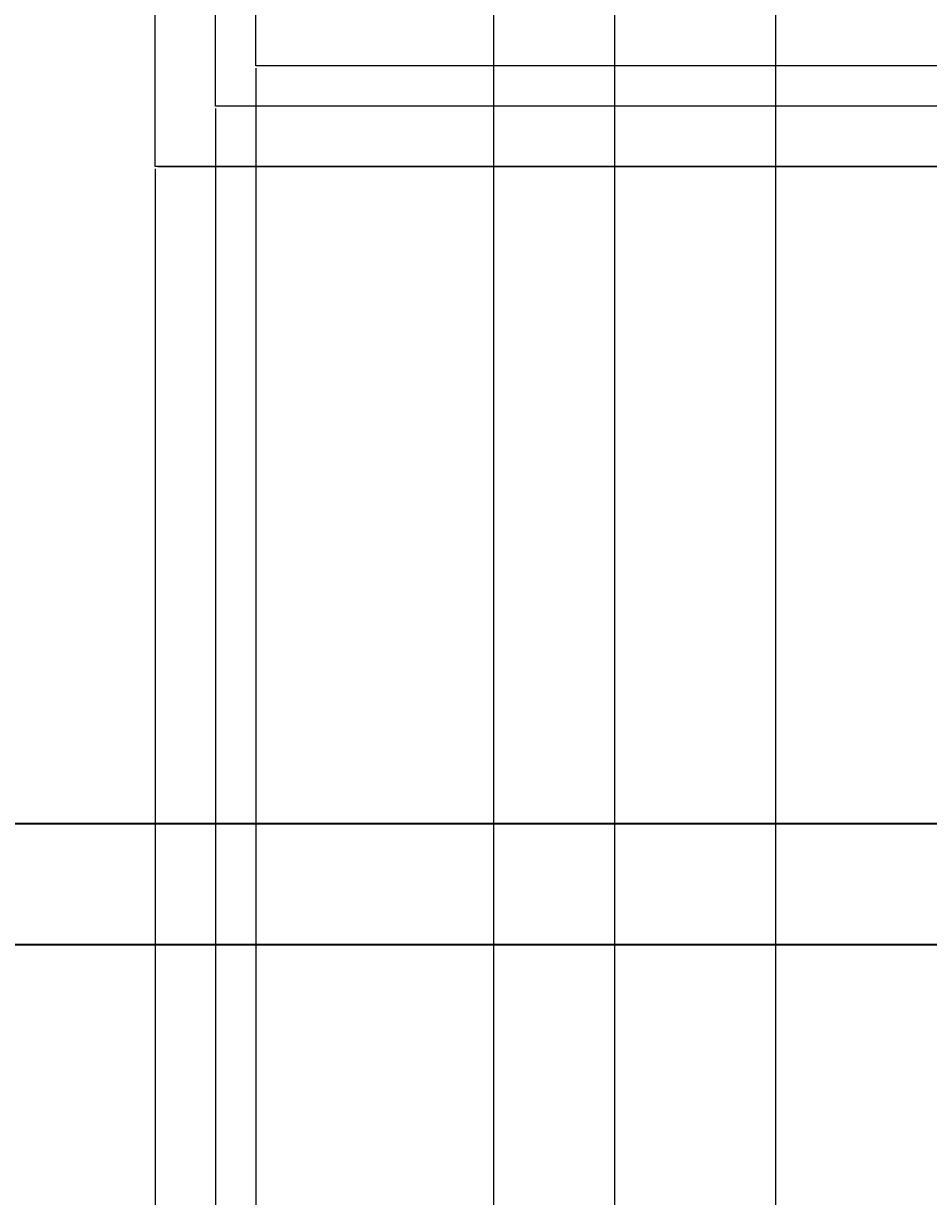
# Model space of a CAD drawing. Units: inches. Extents: x -6 to 289, y -8 to 323.
# Tile 51 of 107: x 124 to 146, y 153 to 182. Entities that reach past the tile are written whole.
import ezdxf

# ---------------------------------------------------------------- set-up
doc = ezdxf.new("R2010")
doc.units = ezdxf.units.IN
doc.header["$MEASUREMENT"] = 0
for name, color, linetype, lineweight in [('A-ANNO-DIMS', 2, 'Continuous', 18), ('A-ELEV', 7, 'Continuous', 35), ('A-ELEV-PATT', 8, 'Continuous', 13), ('A-GLAZ', 4, 'Continuous', 25)]:
    doc.layers.add(name, color=color, linetype=linetype, lineweight=lineweight)
doc.styles.get("Standard").update_dxf_attribs({"font": 'arial.ttf'})
doc.dimstyles.get("Standard").update_dxf_attribs({"dimtxt": 0.18, "dimasz": 0.18, "dimexe": 0.18, "dimexo": 0.0625, "dimgap": 0.09, "dimtad": 0, "dimtih": 1, "dimtoh": 1, "dimdec": 4, "dimzin": 0, "dimdsep": 46, "dimtxsty": 'Standard', "dimcen": 0.09, "dimadec": 0, "dimazin": 0, "dimtfac": 1, "dimtdec": 4, "dimtofl": 0, "dimtmove": 0, "dimatfit": 3, "dimfxl": 1, "dimtolj": 1, "dimtzin": 0, "dimarcsym": 0})

# ---------------------------------------------------------------- blocks, each defined once
blk = doc.blocks.new('*U4')
for p, q in [((1.5, 1.5), (1.5, 46.5)), ((21, 1.5), (1.5, 1.5))]:
    blk.add_line(p, q)
blk.add_lwpolyline([(0, 0), (0, 48), (42, 48), (42, 0)], close=True)
blk.add_lwpolyline([(20, 45.5), (20, 2.5), (2.5, 2.5), (2.5, 45.5), (20, 45.5)])
blk = doc.blocks.new('*D24')
at = {"layer": 'A-ANNO-DIMS', "color": 0, "lineweight": -2, "transparency": 16777216}
for p, q in [((126.946, 178.654), (288.653, 178.654)), ((288.473, 178.474), (288.473, 159.153)), ((288.473, 139.469), (288.473, 158.789)), ((259.226, 139.289), (288.653, 139.289))]:
    blk.add_line(p, q, dxfattribs=at)
at = {"layer": 'A-ANNO-DIMS', "color": 0, "transparency": 16777216}
for points in [[(288.443, 178.474), (288.503, 178.474), (288.473, 178.654)], [(288.443, 139.469), (288.503, 139.469), (288.473, 139.289)]]:
    blk.add_solid(points, dxfattribs=at)
at = {"layer": 'Defpoints', "color": 0, "transparency": 16777216}
for p in [(126.883, 178.654), (288.473, 178.654), (259.164, 139.289)]:
    blk.add_point(p, dxfattribs=at)
at = {"layer": 'A-ANNO-DIMS', "color": 0, "transparency": 16777216, "insert": (288.473, 158.971), "char_height": 0.18, "attachment_point": 5}
blk.add_mtext('\\A1;39.365', dxfattribs=at)
blk = doc.blocks.new('*D25')
at = {"layer": 'A-ANNO-DIMS', "color": 0, "lineweight": -2, "transparency": 16777216}
for p, q in [((126.946, 226.654), (288.653, 226.654)), ((288.473, 226.474), (288.473, 202.836)), ((288.473, 178.834), (288.473, 202.472)), ((126.946, 178.654), (288.653, 178.654))]:
    blk.add_line(p, q, dxfattribs=at)
at = {"layer": 'A-ANNO-DIMS', "color": 0, "transparency": 16777216}
for points in [[(288.443, 226.474), (288.503, 226.474), (288.473, 226.654)], [(288.443, 178.834), (288.503, 178.834), (288.473, 178.654)]]:
    blk.add_solid(points, dxfattribs=at)
at = {"layer": 'Defpoints', "color": 0, "transparency": 16777216}
for p in [(126.883, 226.654), (288.473, 226.654), (126.883, 178.654)]:
    blk.add_point(p, dxfattribs=at)
at = {"layer": 'A-ANNO-DIMS', "color": 0, "transparency": 16777216, "insert": (288.473, 202.654), "char_height": 0.18, "attachment_point": 5}
blk.add_mtext('\\A1;48', dxfattribs=at)
blk = doc.blocks.new('*D28')
at = {"layer": 'A-ANNO-DIMS', "color": 0, "lineweight": -2, "transparency": 16777216}
for p, q in [((128.383, 180.092), (128.383, -8.391)), ((126.883, 178.592), (126.883, -8.391)), ((127.063, -8.211), (127.387, -8.211)), ((128.203, -8.211), (127.88, -8.211))]:
    blk.add_line(p, q, dxfattribs=at)
at = {"layer": 'A-ANNO-DIMS', "color": 0, "transparency": 16777216}
for points in [[(127.063, -8.181), (127.063, -8.241), (126.883, -8.211)], [(128.203, -8.181), (128.203, -8.241), (128.383, -8.211)]]:
    blk.add_solid(points, dxfattribs=at)
at = {"layer": 'Defpoints', "color": 0, "transparency": 16777216}
for p in [(128.383, 180.154), (126.883, 178.654), (128.383, -8.211)]:
    blk.add_point(p, dxfattribs=at)
at = {"layer": 'A-ANNO-DIMS', "color": 0, "transparency": 16777216, "insert": (127.633, -8.211), "char_height": 0.18, "attachment_point": 5}
blk.add_mtext('\\A1;1.5', dxfattribs=at)
blk = doc.blocks.new('*D29')
at = {"layer": 'A-ANNO-DIMS', "color": 0, "lineweight": -2, "transparency": 16777216}
for p, q in [((129.383, 181.092), (129.383, -8.391)), ((128.383, 180.092), (128.383, -8.391)), ((128.563, -8.211), (128.76, -8.211)), ((129.203, -8.211), (129.007, -8.211))]:
    blk.add_line(p, q, dxfattribs=at)
at = {"layer": 'A-ANNO-DIMS', "color": 0, "transparency": 16777216}
for points in [[(128.563, -8.181), (128.563, -8.241), (128.383, -8.211)], [(129.203, -8.181), (129.203, -8.241), (129.383, -8.211)]]:
    blk.add_solid(points, dxfattribs=at)
at = {"layer": 'Defpoints', "color": 0, "transparency": 16777216}
for p in [(129.383, 181.154), (128.383, 180.154), (129.383, -8.211)]:
    blk.add_point(p, dxfattribs=at)
at = {"layer": 'A-ANNO-DIMS', "color": 0, "transparency": 16777216, "insert": (128.883, -8.211), "char_height": 0.18, "attachment_point": 5}
blk.add_mtext('\\A1;1', dxfattribs=at)
blk = doc.blocks.new('*D30')
at = {"layer": 'A-ANNO-DIMS', "color": 0, "lineweight": -2, "transparency": 16777216}
for p, q in [((129.383, 181.092), (129.383, -8.391)), ((146.883, 181.092), (146.883, -8.391)), ((129.563, -8.211), (137.817, -8.211)), ((146.703, -8.211), (138.449, -8.211))]:
    blk.add_line(p, q, dxfattribs=at)
at = {"layer": 'A-ANNO-DIMS', "color": 0, "transparency": 16777216}
for points in [[(129.563, -8.181), (129.563, -8.241), (129.383, -8.211)], [(146.703, -8.181), (146.703, -8.241), (146.883, -8.211)]]:
    blk.add_solid(points, dxfattribs=at)
at = {"layer": 'Defpoints', "color": 0, "transparency": 16777216}
for p in [(129.383, 181.154), (146.883, 181.154), (146.883, -8.211)]:
    blk.add_point(p, dxfattribs=at)
at = {"layer": 'A-ANNO-DIMS', "color": 0, "transparency": 16777216, "insert": (138.133, -8.211), "char_height": 0.18, "attachment_point": 5}
blk.add_mtext('\\A1;17.5', dxfattribs=at)
blk = doc.blocks.new('*D73')
at = {"layer": 'A-ANNO-DIMS', "color": 0, "lineweight": -2, "transparency": 16777216}
for p, q in [((121.008, 51.148), (121.008, 322.969)), ((135.296, 51.148), (135.296, 322.969)), ((121.188, 322.789), (127.697, 322.789)), ((135.116, 322.789), (128.607, 322.789))]:
    blk.add_line(p, q, dxfattribs=at)
at = {"layer": 'A-ANNO-DIMS', "color": 0, "transparency": 16777216}
for points in [[(121.188, 322.819), (121.188, 322.759), (121.008, 322.789)], [(135.116, 322.819), (135.116, 322.759), (135.296, 322.789)]]:
    blk.add_solid(points, dxfattribs=at)
at = {"layer": 'Defpoints', "color": 0, "transparency": 16777216}
for p in [(135.296, 322.789), (121.008, 51.085), (135.296, 51.085)]:
    blk.add_point(p, dxfattribs=at)
at = {"layer": 'A-ANNO-DIMS', "color": 0, "transparency": 16777216, "insert": (128.152, 322.789), "char_height": 0.18, "attachment_point": 5}
blk.add_mtext('\\A1;14.288', dxfattribs=at)
blk = doc.blocks.new('*D74')
at = {"layer": 'A-ANNO-DIMS', "color": 0, "lineweight": -2, "transparency": 16777216}
for p, q in [((135.296, 51.148), (135.296, 322.969)), ((138.296, 51.148), (138.296, 322.969)), ((135.476, 322.789), (136.647, 322.789)), ((138.116, 322.789), (136.945, 322.789))]:
    blk.add_line(p, q, dxfattribs=at)
at = {"layer": 'A-ANNO-DIMS', "color": 0, "transparency": 16777216}
for points in [[(135.476, 322.819), (135.476, 322.759), (135.296, 322.789)], [(138.116, 322.819), (138.116, 322.759), (138.296, 322.789)]]:
    blk.add_solid(points, dxfattribs=at)
at = {"layer": 'Defpoints', "color": 0, "transparency": 16777216}
for p in [(138.296, 322.789), (135.296, 51.085), (138.296, 51.085)]:
    blk.add_point(p, dxfattribs=at)
at = {"layer": 'A-ANNO-DIMS', "color": 0, "transparency": 16777216, "insert": (136.796, 322.789), "char_height": 0.18, "attachment_point": 5}
blk.add_mtext('\\A1;3', dxfattribs=at)
blk = doc.blocks.new('*D75')
at = {"layer": 'A-ANNO-DIMS', "color": 0, "lineweight": -2, "transparency": 16777216}
for p, q in [((138.296, 51.148), (138.296, 322.969)), ((142.296, 51.148), (142.296, 322.969)), ((138.476, 322.789), (140.144, 322.789)), ((142.116, 322.789), (140.448, 322.789))]:
    blk.add_line(p, q, dxfattribs=at)
at = {"layer": 'A-ANNO-DIMS', "color": 0, "transparency": 16777216}
for points in [[(138.476, 322.819), (138.476, 322.759), (138.296, 322.789)], [(142.116, 322.819), (142.116, 322.759), (142.296, 322.789)]]:
    blk.add_solid(points, dxfattribs=at)
at = {"layer": 'Defpoints', "color": 0, "transparency": 16777216}
for p in [(142.296, 322.789), (138.296, 51.085), (142.296, 51.085)]:
    blk.add_point(p, dxfattribs=at)
at = {"layer": 'A-ANNO-DIMS', "color": 0, "transparency": 16777216, "insert": (140.296, 322.789), "char_height": 0.18, "attachment_point": 5}
blk.add_mtext('\\A1;4', dxfattribs=at)
blk = doc.blocks.new('*D76')
at = {"layer": 'A-ANNO-DIMS', "color": 0, "lineweight": -2, "transparency": 16777216}
for p, q in [((142.296, 51.148), (142.296, 322.969)), ((164.296, 51.148), (164.296, 322.969)), ((142.476, 322.789), (153.076, 322.789)), ((164.116, 322.789), (153.516, 322.789))]:
    blk.add_line(p, q, dxfattribs=at)
at = {"layer": 'A-ANNO-DIMS', "color": 0, "transparency": 16777216}
for points in [[(142.476, 322.819), (142.476, 322.759), (142.296, 322.789)], [(164.116, 322.819), (164.116, 322.759), (164.296, 322.789)]]:
    blk.add_solid(points, dxfattribs=at)
at = {"layer": 'Defpoints', "color": 0, "transparency": 16777216}
for p in [(164.296, 322.789), (142.296, 51.085), (164.296, 51.085)]:
    blk.add_point(p, dxfattribs=at)
at = {"layer": 'A-ANNO-DIMS', "color": 0, "transparency": 16777216, "insert": (153.296, 322.789), "char_height": 0.18, "attachment_point": 5}
blk.add_mtext('\\A1;22', dxfattribs=at)
blk = doc.blocks.new('*D94')
at = {"layer": 'A-ANNO-DIMS', "color": 0, "lineweight": -2, "transparency": 16777216}
for p, q in [((118.164, 159.411), (118.164, 322.969)), ((161.552, 159.411), (161.552, 322.969)), ((118.344, 322.789), (139.46, 322.789)), ((161.372, 322.789), (140.256, 322.789))]:
    blk.add_line(p, q, dxfattribs=at)
at = {"layer": 'A-ANNO-DIMS', "color": 0, "transparency": 16777216}
for points in [[(118.344, 322.819), (118.344, 322.759), (118.164, 322.789)], [(161.372, 322.819), (161.372, 322.759), (161.552, 322.789)]]:
    blk.add_solid(points, dxfattribs=at)
at = {"layer": 'Defpoints', "color": 0, "transparency": 16777216}
for p in [(161.552, 322.789), (118.164, 159.348), (161.552, 159.348)]:
    blk.add_point(p, dxfattribs=at)
at = {"layer": 'A-ANNO-DIMS', "color": 0, "transparency": 16777216, "insert": (139.858, 322.789), "char_height": 0.18, "attachment_point": 5}
blk.add_mtext('\\A1;43.39', dxfattribs=at)

msp = doc.modelspace()

# ---------------------------------------------------------------- hatches: boundary and pattern name
at = {"layer": 'A-ELEV-PATT'}
h = msp.add_hatch(dxfattribs=at)
h.set_pattern_fill('_USER', color=256, scale=6, pattern_type=0)
h.set_pattern_definition([(0, (0, 0), (0, 6), [])])
h.paths.add_polyline_path([(184.1244, 48.0851), (124.008, 48.0851), (124.008, 10.2888), (184.1244, 10.2888)])
h.paths.add_polyline_path([(244.2408, 48.0851), (186.3604, 48.0851), (186.3604, 10.2888), (244.2408, 10.2888)])
h.paths.add_polyline_path([(208.2918, 114.2795), (190.7918, 114.2795), (190.7918, 71.2795), (208.2918, 71.2795)])
h.paths.add_polyline_path([(227.7918, 114.2795), (209.2918, 114.2795), (209.2918, 71.2795), (227.7918, 71.2795)])
h.paths.add_polyline_path([(211.2918, 224.3887), (190.7918, 224.3887), (190.7918, 162.3484), (211.2918, 162.3484)])
h.paths.add_polyline_path([(233.7918, 224.3887), (212.2918, 224.3887), (212.2918, 162.3484), (233.7918, 162.3484)])
h.paths.add_polyline_path([(166.3835, 224.154), (147.8835, 224.154), (147.8835, 181.154), (166.3835, 181.154)])
h.paths.add_polyline_path([(146.8835, 224.154), (129.3835, 224.154), (129.3835, 181.154), (146.8835, 181.154)])

# ---------------------------------------------------------------- linework, layer by layer
at = {"layer": 'A-ELEV'}
for points in [[(247.1638, 139.2888), (115.1638, 139.2888), (115.1638, 162.3484), (247.1638, 162.3484)], [(244.1638, 142.2888), (118.1638, 142.2888), (118.1638, 159.3484), (244.1638, 159.3484)]]:
    msp.add_lwpolyline(points, close=True, dxfattribs=at)

# ---------------------------------------------------------------- block references
at = {"layer": 'A-GLAZ'}
msp.add_blockref('*U4', (126.8835, 178.654), dxfattribs=at)

# ---------------------------------------------------------------- dimensions: what is measured, and where the dimension line sits
at = {"layer": 'A-ANNO-DIMS'}
for base, p1, p2, override, picture, middle in [((161.5522, 322.7888), (118.1638, 159.3484), (161.5522, 159.3484), {"dimdec": 2, "dimlfac": 1, "dimrnd": 0, "dimzin": 0, "dimdsep": 46, "dimlunit": 2}, '*D94', (139.858, 322.7888)), ((135.296, 322.7888), (121.008, 51.0851), (135.296, 51.0851), {"dimdec": 3, "dimlfac": 1, "dimrnd": 0, "dimzin": 0, "dimdsep": 46, "dimlunit": 2}, '*D73', (128.152, 322.7888)), ((138.296, 322.7888), (135.296, 51.0851), (138.296, 51.0851), {"dimdec": 0, "dimlfac": 1, "dimrnd": 0, "dimzin": 0, "dimdsep": 46, "dimlunit": 2}, '*D74', (136.796, 322.7888)), ((142.296, 322.7888), (138.296, 51.0851), (142.296, 51.0851), {"dimdec": 0, "dimlfac": 1, "dimrnd": 0, "dimzin": 0, "dimdsep": 46, "dimlunit": 2}, '*D75', (140.296, 322.7888)), ((164.296, 322.7888), (142.296, 51.0851), (164.296, 51.0851), {"dimdec": 0, "dimlfac": 1, "dimrnd": 0, "dimzin": 0, "dimdsep": 46, "dimlunit": 2}, '*D76', (153.296, 322.7888)), ((129.3835, -8.2112), (128.3835, 180.154), (129.3835, 181.154), {"dimdec": 0, "dimlfac": 1, "dimrnd": 0, "dimzin": 0, "dimdsep": 46, "dimlunit": 2}, '*D29', (128.8835, -8.2112)), ((146.8835, -8.2112), (129.3835, 181.154), (146.8835, 181.154), {"dimdec": 1, "dimlfac": 1, "dimrnd": 0, "dimzin": 0, "dimdsep": 46, "dimlunit": 2}, '*D30', (138.1335, -8.2112)), ((128.3835, -8.2112), (126.8835, 178.654), (128.3835, 180.154), {"dimdec": 1, "dimlfac": 1, "dimrnd": 0, "dimzin": 0, "dimdsep": 46, "dimlunit": 2}, '*D28', (127.6335, -8.2112))]:
    dim = msp.add_linear_dim(base=base, p1=p1, p2=p2, dimstyle='Standard', override=override, dxfattribs=at)
    dim.commit()
    dim.dimension.update_dxf_attribs({"geometry": picture, "text_midpoint": middle})
for base, p1, p2, override, picture, middle in [((288.4733, 226.654), (126.8835, 178.654), (126.8835, 226.654), {"dimdec": 0, "dimlfac": 1, "dimrnd": 0, "dimzin": 0, "dimdsep": 46, "dimlunit": 2}, '*D25', (288.4733, 202.654)), ((288.4733, 178.654), (259.1638, 139.2888), (126.8835, 178.654), {"dimdec": 3, "dimlfac": 1, "dimrnd": 0, "dimzin": 0, "dimdsep": 46, "dimlunit": 2}, '*D24', (288.4733, 158.9714))]:
    dim = msp.add_linear_dim(base=base, p1=p1, p2=p2, angle=90, dimstyle='Standard', override=override, dxfattribs=at)
    dim.commit()
    dim.dimension.update_dxf_attribs({"geometry": picture, "text_midpoint": middle})

doc.saveas('drawing.dxf')
